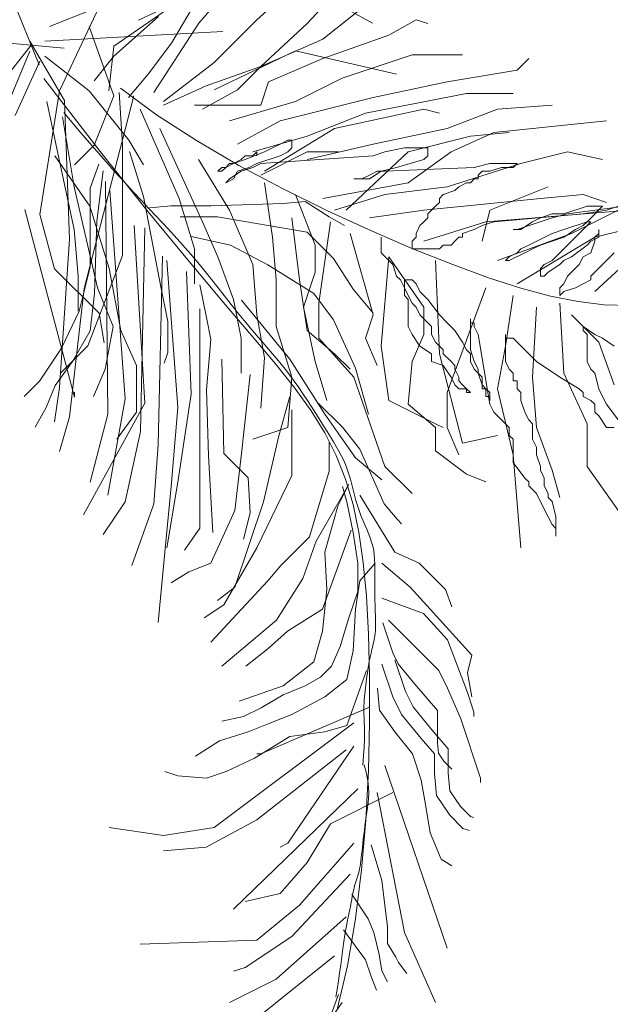
# Model space of a CAD drawing. Units: millimetres. Extents: x 595116 to 630915, y 909473 to 920225.
# Tile 98 of 134: x 629805.265 to 629809.617, y 919164.766 to 919172.019. Entities that reach past the tile are written whole.
import ezdxf

# ---------------------------------------------------------------- set-up
doc = ezdxf.new("R2010")
doc.units = ezdxf.units.MM
doc.layers.add('L-PLNT', color=85, linetype='Continuous', lineweight=13)

# ---------------------------------------------------------------- blocks, each defined once
blk = doc.blocks.new('A$C4FB75ABC')
for p, q in [((2.6324, 2.4053), (2.7073, 2.2214)), ((3.0207, 2.3031), (3.1093, 2.4053)), ((3.1344, 2.3096), (3.2259, 2.3934)), ((3.2335, 2.302), (3.3174, 2.3934)), ((2.7277, 2.2964), (2.8733, 2.3546)), ((2.8539, 2.2576), (2.9801, 2.3449)), ((2.9022, 2.3089), (3.0036, 2.3566)), ((2.9666, 2.2638), (3.0123, 2.3401)), ((2.8248, 2.3352), (2.7471, 2.1703)), ((3.264, 2.2715), (3.3403, 2.3324)), ((3.3079, 2.3327), (3.3615, 2.3029)), ((2.8539, 2.2382), (2.9413, 2.3158)), ((2.9321, 2.167), (3.0207, 2.3031)), ((3.0505, 2.2257), (3.1344, 2.3096)), ((3.142, 2.2181), (3.2335, 2.302)), ((3.3937, 2.2791), (3.447, 2.3096)), ((3.447, 2.3096), (3.4699, 2.302)), ((2.718, 2.2673), (3.0675, 2.2867)), ((2.8054, 2.2964), (2.8539, 2.1606)), ((2.6937, 2.2623), (2.4825, 1.9967)), ((2.7559, 2.2536), (2.4852, 2.2785)), ((2.6889, 2.2673), (2.7568, 2.1509)), ((2.9208, 2.2029), (2.9666, 2.2638)), ((3.142, 2.2181), (3.264, 2.2715)), ((3.264, 2.2334), (3.3937, 2.2791)), ((2.6889, 2.2479), (2.6404, 2.1315)), ((2.8442, 2.1703), (2.8539, 2.2576)), ((3.0505, 2.1724), (3.2106, 2.2486)), ((3.2106, 2.2486), (3.4089, 2.2029)), ((2.7083, 2.2285), (2.6598, 2.1218)), ((2.718, 2.2382), (2.8054, 2.1703)), ((2.8151, 2.1897), (2.8539, 2.2382)), ((2.9513, 2.1495), (3.0505, 2.2257)), ((3.1572, 2.1876), (3.264, 2.2334)), ((3.3021, 2.1952), (3.4394, 2.241)), ((3.4394, 2.241), (3.5385, 2.241)), ((3.6453, 2.2105), (3.6682, 2.2334)), ((3.0352, 2.18), (3.142, 2.2181)), ((3.0962, 2.1724), (3.142, 2.2181)), ((3.508, 2.1876), (3.6453, 2.2105)), ((2.7162, 2.1941), (2.8268, 2.0511)), ((2.8827, 2.1571), (2.9208, 2.2029)), ((3.142, 2.1419), (3.1572, 2.1876)), ((3.2106, 2.1495), (3.3021, 2.1952)), ((3.3631, 2.1571), (3.508, 2.1876)), ((2.7471, 2.1703), (2.7083, 1.9277)), ((2.8054, 2.1703), (2.883, 2.0733)), ((2.864, 2.167), (2.8708, 2.0648)), ((2.9375, 2.1232), (2.8667, 2.1755)), ((2.9513, 2.1419), (3.0352, 2.18)), ((3.0276, 2.1343), (3.0962, 2.1724)), ((3.3479, 2.1266), (3.5462, 2.1648)), ((3.5462, 2.1648), (3.6377, 2.1648)), ((2.7225, 2.1495), (2.753, 2.0047)), ((2.7568, 2.1509), (2.7666, 1.8792)), ((2.8927, 2.1606), (2.7957, 1.7822)), ((2.8539, 2.1606), (2.8151, 2.0636)), ((3.081, 2.1114), (3.2106, 2.1495)), ((3.1801, 2.1114), (3.3631, 2.1571)), ((2.7555, 2.1274), (2.7844, 2.0931)), ((2.9056, 2.1343), (2.9818, 1.9589)), ((3.0123, 2.1419), (3.142, 2.1419)), ((3.2335, 2.0809), (3.3479, 2.1266)), ((3.2869, 2.0961), (3.4623, 2.1343)), ((3.4623, 2.1343), (3.4928, 2.1266)), ((3.508, 2.0961), (3.6072, 2.1343)), ((3.6072, 2.1343), (3.714, 2.1419)), ((2.753, 2.119), (2.7759, 1.9818)), ((3.0158, 2.0725), (2.9375, 2.1232)), ((3.0962, 2.0657), (3.1801, 2.1114)), ((3.5996, 2.0885), (3.8207, 2.1114)), ((2.7844, 2.0931), (2.8104, 2.0628)), ((2.9437, 2.0961), (3.0276, 1.9132)), ((3.1496, 2.0123), (3.2869, 2.0961)), ((3.3631, 2.0657), (3.508, 2.0961)), ((3.5157, 2.0504), (3.5996, 2.0885)), ((3.5538, 2.0809), (3.6301, 2.0885)), ((2.883, 2.0733), (2.9122, 2.0248)), ((3.0992, 2.0238), (3.0158, 2.0725)), ((3.1267, 2.0504), (3.2335, 2.0809)), ((3.1954, 2.0733), (3.1801, 2.0657)), ((3.203, 2.0733), (3.1954, 2.0733)), ((3.203, 2.058), (3.203, 2.0733)), ((3.4318, 2.0504), (3.5538, 2.0809)), ((2.8151, 2.0636), (2.7763, 2.0248)), ((2.8104, 2.0628), (2.8339, 2.0359)), ((2.8268, 2.0511), (2.9214, 1.9326)), ((2.8708, 2.0648), (2.8708, 1.8469)), ((2.8844, 2.0512), (2.9117, 1.9627)), ((3.1496, 2.0504), (3.1115, 2.0352)), ((3.1267, 2.0428), (3.1344, 2.0504)), ((3.1344, 2.0504), (3.1344, 2.0428)), ((3.142, 2.0047), (3.2335, 2.0504)), ((3.1649, 2.058), (3.1496, 2.0504)), ((3.1801, 2.0657), (3.1649, 2.058)), ((3.1801, 2.0428), (3.1954, 2.0504)), ((3.1954, 2.0504), (3.203, 2.058)), ((3.2335, 2.0352), (3.3631, 2.0657)), ((3.2335, 2.0504), (3.2945, 2.0504)), ((3.3098, 1.9361), (3.4318, 2.0504)), ((3.386, 2.0504), (3.3631, 2.0428)), ((3.4242, 2.058), (3.386, 2.0504)), ((3.4699, 2.058), (3.4242, 2.058)), ((3.4318, 1.9894), (3.5157, 2.0504)), ((3.4699, 2.0428), (3.4699, 2.058)), ((3.6529, 2.0275), (3.7445, 2.0504)), ((3.7445, 2.0504), (3.8131, 2.0352)), ((2.7378, 2.0428), (2.8064, 1.9437)), ((2.8339, 2.0359), (2.8551, 2.0121)), ((3.02, 2.0352), (3.081, 1.9361)), ((3.1115, 2.0352), (3.0886, 2.0275)), ((3.0886, 2.0275), (3.1039, 2.0352)), ((3.1039, 2.0352), (3.1115, 2.0428)), ((3.1115, 2.0428), (3.1267, 2.0428)), ((3.1344, 2.0275), (3.1801, 2.0428)), ((3.3631, 2.0428), (3.142, 2.0275)), ((3.4089, 2.0199), (3.4623, 2.0352)), ((3.4623, 2.0352), (3.4699, 2.0428)), ((2.8244, 2.0263), (2.8071, 1.979)), ((2.833, 2.0134), (2.8201, 1.9144)), ((2.8551, 2.0121), (2.8744, 1.9909)), ((3.0581, 2.0123), (3.0657, 2.0199)), ((3.0657, 2.0123), (3.0581, 2.0123)), ((3.0734, 2.0199), (3.0657, 2.0123)), ((3.0657, 2.0199), (3.0734, 2.0199)), ((3.0734, 2.0199), (3.081, 2.0275)), ((3.0886, 2.0275), (3.0734, 2.0199)), ((3.081, 2.0275), (3.0886, 2.0275)), ((3.1039, 2.0123), (3.081, 1.9971)), ((3.0886, 1.9971), (3.0962, 2.0123)), ((3.0962, 2.0123), (3.1191, 2.0199)), ((3.1858, 1.9776), (3.0992, 2.0238)), ((3.1267, 2.0199), (3.1039, 2.0123)), ((3.1191, 2.0199), (3.1344, 2.0275)), ((3.142, 2.0275), (3.1267, 2.0199)), ((3.3708, 2.0123), (3.3555, 2.0047)), ((3.3555, 1.9971), (3.3784, 2.0123)), ((3.386, 2.0123), (3.3708, 2.0123)), ((3.3784, 2.0123), (3.4089, 2.0199)), ((3.5614, 2.0199), (3.386, 2.0123)), ((3.508, 1.9818), (3.6529, 2.0275)), ((3.5919, 2.0275), (3.5614, 2.0199)), ((3.5691, 2.0047), (3.5767, 2.0123)), ((3.5767, 2.0123), (3.5919, 2.0123)), ((3.6453, 2.0275), (3.5919, 2.0275)), ((3.5919, 2.0123), (3.6148, 2.0199)), ((3.6148, 2.0199), (3.6377, 2.0199)), ((3.6377, 2.0199), (3.6453, 2.0275)), ((2.753, 2.0047), (2.7759, 1.898)), ((2.8373, 1.9919), (2.8416, 1.5357)), ((2.8744, 1.9909), (2.8918, 1.9721)), ((3.081, 1.9971), (3.0734, 1.9894)), ((3.0734, 1.9894), (3.0886, 1.9971)), ((3.3403, 1.9971), (3.325, 1.9971)), ((3.325, 1.9971), (3.3555, 1.9971)), ((3.3555, 2.0047), (3.3403, 1.9971)), ((3.5538, 1.9894), (3.5614, 1.9971)), ((3.5614, 1.9971), (3.5691, 1.9971)), ((3.5691, 1.9971), (3.5691, 2.0047)), ((2.7759, 1.9818), (2.8217, 1.7836)), ((2.8071, 1.979), (2.8071, 1.9015)), ((2.8459, 1.9747), (2.876, 1.5659)), ((2.8918, 1.9721), (2.9078, 1.955)), ((3.1496, 1.9894), (3.1649, 1.8827)), ((3.2732, 1.9345), (3.1858, 1.9776)), ((3.264, 1.9589), (3.4318, 1.9894)), ((3.386, 1.9666), (3.508, 1.9818)), ((3.5004, 1.9666), (3.5233, 1.9742)), ((3.5233, 1.9742), (3.5309, 1.9818)), ((3.5309, 1.9818), (3.5462, 1.9894)), ((3.5462, 1.9894), (3.5538, 1.9894)), ((3.5919, 1.9361), (3.7063, 1.9818)), ((2.9078, 1.955), (2.9225, 1.9395)), ((2.9117, 1.9627), (2.9458, 1.7856)), ((2.9818, 1.9589), (3.0123, 1.8599)), ((3.186, 1.9488), (3.2291, 1.9531)), ((3.2106, 1.9666), (3.2488, 1.8675)), ((3.2291, 1.9531), (3.2764, 1.923)), ((3.2869, 1.9361), (3.386, 1.9666)), ((3.4623, 1.9361), (3.6911, 1.9589)), ((3.4928, 1.9589), (3.5004, 1.9666)), ((3.4928, 1.9513), (3.4928, 1.9589)), ((3.6911, 1.9589), (3.775, 1.9666)), ((3.7521, 1.8903), (3.8894, 1.9589)), ((3.775, 1.9666), (3.8207, 1.9513)), ((2.6792, 1.9375), (2.7763, 1.5688)), ((2.8064, 1.9437), (2.8446, 1.8217)), ((2.9214, 1.9326), (3.0014, 1.8351)), ((2.9225, 1.9395), (2.9361, 1.925)), ((2.9234, 1.9402), (2.9664, 1.9445)), ((2.9664, 1.9445), (3.0439, 1.9445)), ((3.0439, 1.9445), (3.186, 1.9488)), ((3.081, 1.9361), (3.1267, 1.8294)), ((3.3593, 1.8951), (3.2732, 1.9345)), ((3.3555, 1.9208), (3.4623, 1.9361)), ((3.4699, 1.9285), (3.4852, 1.9437)), ((3.4852, 1.9437), (3.4928, 1.9513)), ((3.5767, 1.8751), (3.5919, 1.9361)), ((3.5843, 1.9132), (3.8665, 1.9361)), ((3.7826, 1.9437), (3.7368, 1.9285)), ((3.7445, 1.9285), (3.9122, 1.9513)), ((3.8207, 1.9361), (3.775, 1.9285)), ((3.7826, 1.9132), (3.8131, 1.9437)), ((3.8131, 1.9437), (3.7826, 1.9437)), ((3.7978, 1.8827), (4.0495, 1.9437)), ((3.8665, 1.9513), (3.8207, 1.9361)), ((2.7083, 1.9277), (2.7374, 1.821)), ((2.8201, 1.9144), (2.8158, 1.7724)), ((2.9361, 1.925), (2.9489, 1.9114)), ((2.9837, 1.923), (3.0569, 1.923)), ((3.0276, 1.9132), (3.0581, 1.8446)), ((3.0569, 1.923), (3.2334, 1.8929)), ((3.203, 1.9208), (3.2182, 1.7989)), ((3.2793, 1.9132), (3.2564, 1.7531)), ((3.2764, 1.923), (3.3066, 1.9058)), ((3.4547, 1.9056), (3.4623, 1.9132)), ((3.4623, 1.9132), (3.4699, 1.9208)), ((3.4623, 1.8751), (3.5843, 1.9132)), ((3.4699, 1.9208), (3.4699, 1.9285)), ((3.5996, 1.9132), (3.5767, 1.9056)), ((3.775, 1.9285), (3.5996, 1.9132)), ((3.6453, 1.898), (3.714, 1.9208)), ((3.6758, 1.9132), (3.6529, 1.898)), ((3.6911, 1.9208), (3.6758, 1.9132)), ((3.714, 1.9285), (3.6911, 1.9208)), ((3.7368, 1.9285), (3.714, 1.9285)), ((3.714, 1.9208), (3.7445, 1.9285)), ((3.7368, 1.898), (3.7826, 1.9132)), ((3.7826, 1.9132), (3.775, 1.9056)), ((3.7826, 1.9056), (3.7902, 1.9132)), ((3.7902, 1.9132), (3.7826, 1.9132)), ((2.7759, 1.898), (2.7836, 1.8065)), ((2.8071, 1.9015), (2.8071, 1.8241)), ((2.8933, 1.9058), (2.9148, 1.5573)), ((2.9148, 1.9015), (2.9062, 1.5013)), ((2.9489, 1.9114), (2.9609, 1.8985)), ((2.9609, 1.8985), (2.9724, 1.8861)), ((3.4421, 1.8597), (3.3593, 1.8951)), ((3.447, 1.8903), (3.4547, 1.9056)), ((3.5614, 1.898), (3.5385, 1.8903)), ((3.5767, 1.9056), (3.5614, 1.898)), ((3.6529, 1.898), (3.6377, 1.898)), ((3.6377, 1.898), (3.6453, 1.898)), ((3.714, 1.8903), (3.7368, 1.898)), ((3.7597, 1.898), (3.7368, 1.8827)), ((3.7597, 1.8827), (3.7826, 1.9056)), ((3.775, 1.9056), (3.7597, 1.898)), ((3.8055, 1.8903), (3.8055, 1.898)), ((3.8055, 1.898), (3.8055, 1.8827)), ((2.7666, 1.8792), (2.7471, 1.5882)), ((2.9724, 1.8861), (2.9834, 1.874)), ((3.0052, 1.8843), (3.0827, 1.8671)), ((3.1649, 1.8827), (3.1725, 1.7989)), ((3.2334, 1.8929), (3.285, 1.8413)), ((3.3174, 1.8903), (3.3631, 1.7303)), ((3.3784, 1.8827), (3.3784, 1.8522)), ((3.4394, 1.8751), (3.447, 1.8827)), ((3.4394, 1.8599), (3.4394, 1.8751)), ((3.447, 1.8827), (3.447, 1.8903)), ((3.5233, 1.8751), (3.5157, 1.8675)), ((3.5309, 1.8827), (3.5233, 1.8751)), ((3.5385, 1.8827), (3.5309, 1.8827)), ((3.5385, 1.8903), (3.5385, 1.8827)), ((3.6072, 1.837), (3.7521, 1.8903)), ((3.6453, 1.7913), (3.7978, 1.8827)), ((3.6682, 1.8675), (3.714, 1.8903)), ((3.7368, 1.8827), (3.6911, 1.8675)), ((3.7368, 1.8599), (3.7521, 1.8751)), ((3.7521, 1.8751), (3.7597, 1.8827)), ((3.7902, 1.8751), (3.7826, 1.8675)), ((3.8055, 1.8827), (3.7902, 1.8751)), ((3.7902, 1.8522), (3.7978, 1.8751)), ((3.7978, 1.8827), (3.8055, 1.8903)), ((3.7978, 1.8751), (3.7978, 1.8827)), ((2.9834, 1.874), (2.994, 1.862)), ((2.994, 1.862), (3.0045, 1.8499)), ((3.0123, 1.8599), (3.0123, 1.7913)), ((3.0827, 1.8671), (3.1559, 1.8284)), ((3.2488, 1.8675), (3.2488, 1.8141)), ((3.4928, 1.8599), (3.4394, 1.8599)), ((3.5192, 1.829), (3.4421, 1.8597)), ((3.5004, 1.8675), (3.4928, 1.8599)), ((3.5157, 1.8675), (3.5004, 1.8675)), ((3.6453, 1.8522), (3.6529, 1.8599)), ((3.6529, 1.8599), (3.6682, 1.8675)), ((3.6758, 1.8599), (3.6606, 1.8522)), ((3.6911, 1.8675), (3.6758, 1.8599)), ((3.714, 1.837), (3.7368, 1.8599)), ((3.7826, 1.8675), (3.7521, 1.8446)), ((3.7978, 1.776), (3.897, 1.8675)), ((2.8708, 1.8469), (2.8027, 1.6699)), ((2.9492, 1.8456), (2.9406, 1.4755)), ((2.9578, 1.837), (2.9794, 1.5486)), ((3.0045, 1.8499), (3.0149, 1.8377)), ((3.0149, 1.8377), (3.0253, 1.8251)), ((3.0581, 1.8446), (3.0886, 1.7608)), ((3.285, 1.8413), (3.3238, 1.781)), ((3.3784, 1.8522), (3.3937, 1.837)), ((3.3937, 1.8446), (3.3784, 1.6693)), ((3.3937, 1.8446), (3.4623, 1.7455)), ((3.3937, 1.837), (3.4013, 1.8294)), ((3.4852, 1.837), (3.4928, 1.6541)), ((3.6224, 1.837), (3.6301, 1.8446)), ((3.6301, 1.837), (3.6224, 1.837)), ((3.6606, 1.8522), (3.6301, 1.837)), ((3.6301, 1.8446), (3.6453, 1.8522)), ((3.6987, 1.8294), (3.714, 1.837)), ((3.7368, 1.837), (3.7292, 1.8294)), ((3.7521, 1.8446), (3.7368, 1.837)), ((3.7673, 1.8294), (3.775, 1.8446)), ((3.775, 1.8446), (3.7902, 1.8522)), ((3.8207, 1.837), (3.8131, 1.8294)), ((3.836, 1.8522), (3.8207, 1.837)), ((2.7374, 1.821), (2.8248, 1.7337)), ((2.8071, 1.8241), (2.7856, 1.738)), ((2.8446, 1.8217), (2.8674, 1.6998)), ((3.0014, 1.8351), (3.0686, 1.7552)), ((3.0253, 1.8251), (3.0358, 1.8122)), ((3.1267, 1.8294), (3.1344, 1.7303)), ((3.1559, 1.8284), (3.2463, 1.7724)), ((3.4013, 1.8294), (3.4089, 1.8065)), ((3.5892, 1.8034), (3.5192, 1.829)), ((3.6911, 1.8217), (3.6987, 1.8294)), ((3.6911, 1.8065), (3.6911, 1.8217)), ((3.7292, 1.8294), (3.7063, 1.8141)), ((3.7445, 1.8065), (3.7673, 1.8294)), ((3.8131, 1.8294), (3.7902, 1.8065)), ((2.7836, 1.8065), (2.7836, 1.7379)), ((2.9966, 1.8154), (3.0052, 1.5745)), ((3.0358, 1.8122), (3.0461, 1.7993)), ((3.0461, 1.7993), (3.0562, 1.7866)), ((3.1725, 1.7989), (3.1725, 1.7074)), ((3.2182, 1.7989), (3.2335, 1.6998)), ((3.2488, 1.8141), (3.2259, 1.7455)), ((3.4089, 1.8065), (3.4165, 1.7989)), ((3.4165, 1.7989), (3.4242, 1.7836)), ((3.4242, 1.7684), (3.4242, 1.7989)), ((3.4242, 1.7989), (3.4394, 1.7989)), ((3.4394, 1.7989), (3.447, 1.7913)), ((3.6527, 1.7828), (3.5892, 1.8034)), ((3.6987, 1.8065), (3.6911, 1.8065)), ((3.7063, 1.8141), (3.6987, 1.8065)), ((3.7368, 1.7913), (3.7445, 1.8065)), ((3.7902, 1.7989), (3.775, 1.7913)), ((3.7902, 1.8065), (3.7902, 1.7989)), ((2.7957, 1.7822), (2.7666, 1.53)), ((2.8217, 1.7836), (2.8522, 1.7074)), ((2.9458, 1.7856), (2.9594, 1.7175)), ((3.0224, 1.7896), (3.0353, 1.7251)), ((3.0562, 1.7866), (3.0659, 1.7741)), ((3.3238, 1.781), (3.3625, 1.7337)), ((3.4242, 1.7836), (3.4318, 1.7684)), ((3.447, 1.7913), (3.4547, 1.776)), ((3.5843, 1.7836), (3.508, 1.5778)), ((3.7109, 1.7672), (3.6527, 1.7828)), ((3.7292, 1.7836), (3.7368, 1.7913)), ((3.7292, 1.7684), (3.7292, 1.7836)), ((3.7597, 1.7836), (3.7368, 1.776)), ((3.775, 1.7913), (3.7597, 1.7836)), ((2.8158, 1.7724), (2.8071, 1.6993)), ((3.0659, 1.7741), (3.0752, 1.7623)), ((3.0752, 1.7623), (3.084, 1.7511)), ((3.0886, 1.7608), (3.1039, 1.6845)), ((3.1042, 1.7595), (3.1989, 1.6433)), ((3.2463, 1.7724), (3.285, 1.7208)), ((3.4318, 1.7608), (3.4242, 1.7684)), ((3.4318, 1.7684), (3.4394, 1.7531)), ((3.4318, 1.7074), (3.4318, 1.7608)), ((3.4547, 1.776), (3.4699, 1.7608)), ((3.4699, 1.7608), (3.4928, 1.7303)), ((3.6377, 1.7684), (3.6224, 1.6693)), ((3.7651, 1.7564), (3.7109, 1.7672)), ((3.7368, 1.776), (3.7292, 1.7684)), ((3.0224, 1.7423), (3.0224, 1.312)), ((3.0686, 1.7552), (3.1246, 1.6894)), ((3.084, 1.7511), (3.0921, 1.7408)), ((3.0921, 1.7408), (3.0994, 1.7316)), ((3.2259, 1.7455), (3.2488, 1.6388)), ((3.2564, 1.7531), (3.2564, 1.6845)), ((3.4394, 1.7531), (3.447, 1.7455)), ((3.447, 1.7455), (3.4547, 1.7303)), ((3.4623, 1.7455), (3.4623, 1.6922)), ((3.6834, 1.7455), (3.6758, 1.6083)), ((3.7292, 1.7531), (3.7368, 1.6159)), ((3.8165, 1.7504), (3.7651, 1.7564)), ((3.8664, 1.749), (3.8165, 1.7504)), ((2.7856, 1.738), (2.7512, 1.6648)), ((2.8248, 1.7337), (2.8345, 1.6755)), ((3.0353, 1.7251), (3.0439, 1.682)), ((3.0994, 1.7316), (3.1062, 1.7232)), ((3.1062, 1.7232), (3.1126, 1.7155)), ((3.1344, 1.7303), (3.1496, 1.6464)), ((3.285, 1.7208), (3.3281, 1.6261)), ((3.3631, 1.7303), (3.3479, 1.6845)), ((3.4547, 1.7303), (3.4699, 1.715)), ((3.4928, 1.7303), (3.508, 1.715)), ((3.5538, 1.7227), (3.5538, 1.715)), ((3.5538, 1.6617), (3.5538, 1.7227)), ((3.7521, 1.7303), (3.8055, 1.6769)), ((2.8522, 1.7074), (2.8369, 1.6236)), ((2.9594, 1.7175), (2.9594, 1.6563)), ((3.1126, 1.7155), (3.1186, 1.7083)), ((3.1186, 1.7083), (3.1246, 1.7013)), ((3.1246, 1.7013), (3.1305, 1.6944)), ((3.1725, 1.7074), (3.203, 1.6083)), ((3.4394, 1.6922), (3.4318, 1.7074)), ((3.4699, 1.715), (3.4775, 1.7074)), ((3.4775, 1.7074), (3.4775, 1.6922)), ((3.508, 1.715), (3.5233, 1.6998)), ((3.5538, 1.715), (3.5614, 1.715)), ((3.5614, 1.715), (3.5614, 1.7074)), ((3.5614, 1.7074), (3.5691, 1.6922)), ((3.775, 1.6998), (3.775, 1.7074)), ((3.775, 1.7074), (3.7978, 1.6922)), ((2.8071, 1.6993), (2.7727, 1.639)), ((2.8674, 1.6998), (2.8979, 1.6312)), ((3.0439, 1.682), (3.0353, 1.5831)), ((3.1039, 1.6845), (3.1039, 1.6159)), ((3.1246, 1.6894), (3.1709, 1.6342)), ((3.1305, 1.6944), (3.1367, 1.6873)), ((3.1367, 1.6873), (3.1432, 1.6798)), ((3.2335, 1.6998), (3.2869, 1.6541)), ((3.2564, 1.6845), (3.325, 1.6083)), ((3.3479, 1.6845), (3.3708, 1.6312)), ((3.4547, 1.6693), (3.4394, 1.6922)), ((3.4623, 1.6922), (3.4394, 1.6388)), ((3.4775, 1.6922), (3.4852, 1.6769)), ((3.5233, 1.6998), (3.5385, 1.6769)), ((3.5691, 1.6922), (3.5919, 1.555)), ((3.6224, 1.6922), (3.6224, 1.6845)), ((3.6224, 1.6388), (3.6224, 1.6922)), ((3.6224, 1.6845), (3.6377, 1.6845)), ((3.6377, 1.6845), (3.6453, 1.6769)), ((3.7826, 1.6922), (3.775, 1.6998)), ((3.7826, 1.6388), (3.7826, 1.6922)), ((3.7978, 1.6922), (3.8131, 1.6845)), ((3.8131, 1.6845), (3.836, 1.6693)), ((2.7512, 1.6648), (2.7081, 1.6003)), ((2.8027, 1.6699), (2.7482, 1.6154)), ((3.1432, 1.6798), (3.1502, 1.6718)), ((3.1502, 1.6718), (3.1576, 1.6632)), ((3.1576, 1.6632), (3.1654, 1.654)), ((3.3784, 1.6693), (3.3937, 1.5626)), ((3.4775, 1.6541), (3.4547, 1.6693)), ((3.4852, 1.6769), (3.4928, 1.6693)), ((3.4928, 1.6693), (3.5004, 1.6617)), ((3.5385, 1.6769), (3.5462, 1.6617)), ((3.6224, 1.6693), (3.6072, 1.5855)), ((3.6453, 1.6769), (3.6682, 1.6541)), ((3.8055, 1.6769), (3.836, 1.5931)), ((2.9594, 1.6563), (2.9526, 1.6358)), ((3.0655, 1.6433), (3.0698, 1.4583)), ((3.1496, 1.6464), (3.142, 1.5473)), ((3.1654, 1.654), (3.1735, 1.6443)), ((3.1735, 1.6443), (3.1819, 1.634)), ((3.1989, 1.6433), (3.2678, 1.5357)), ((3.2869, 1.6541), (3.3174, 1.6236)), ((3.4775, 1.6388), (3.4775, 1.6541)), ((3.4928, 1.6541), (3.5385, 1.4787)), ((3.5004, 1.6617), (3.5004, 1.6541)), ((3.5004, 1.6541), (3.5157, 1.6388)), ((3.5462, 1.6617), (3.5538, 1.6541)), ((3.5614, 1.6388), (3.5538, 1.6617)), ((3.5538, 1.6541), (3.5538, 1.6388)), ((3.6682, 1.6541), (3.6834, 1.6388)), ((2.7727, 1.639), (2.7383, 1.5917)), ((2.8369, 1.6236), (2.8141, 1.5702)), ((2.8979, 1.6312), (2.8979, 1.5397)), ((3.1709, 1.6342), (3.2091, 1.5863)), ((3.1819, 1.634), (3.1904, 1.6232)), ((3.2488, 1.6388), (3.2716, 1.5626)), ((3.3281, 1.6261), (3.3539, 1.5357)), ((3.4394, 1.6388), (3.4318, 1.555)), ((3.5004, 1.6312), (3.4775, 1.6388)), ((3.5157, 1.6083), (3.5004, 1.6312)), ((3.5157, 1.6388), (3.5233, 1.6312)), ((3.5233, 1.6312), (3.5233, 1.6236)), ((3.5233, 1.6236), (3.5309, 1.6083)), ((3.5538, 1.6388), (3.5614, 1.6236)), ((3.5691, 1.6236), (3.5614, 1.6388)), ((3.5614, 1.6236), (3.5691, 1.6159)), ((3.5691, 1.6159), (3.5691, 1.6236)), ((3.6301, 1.6236), (3.6224, 1.6388)), ((3.6377, 1.6159), (3.6301, 1.6236)), ((3.6834, 1.6388), (3.7292, 1.6083)), ((3.7902, 1.6236), (3.7826, 1.6388)), ((3.7978, 1.6159), (3.7902, 1.6236)), ((3.1214, 1.6132), (3.1042, 1.4583)), ((3.1904, 1.6232), (3.1991, 1.6119)), ((3.203, 1.6083), (3.1954, 1.5092)), ((3.1991, 1.6119), (3.2078, 1.6)), ((3.325, 1.6083), (3.386, 1.433)), ((3.5233, 1.5931), (3.5157, 1.6083)), ((3.5309, 1.6083), (3.5309, 1.6007)), ((3.5691, 1.6159), (3.5767, 1.6083)), ((3.5767, 1.5931), (3.5691, 1.6159)), ((3.5767, 1.6083), (3.5767, 1.5855)), ((3.6377, 1.6007), (3.6377, 1.6159)), ((3.6758, 1.6083), (3.6834, 1.5092)), ((3.7292, 1.6083), (3.7673, 1.5855)), ((3.7368, 1.6159), (3.7826, 1.5168)), ((3.8055, 1.5855), (3.7978, 1.6159)), ((2.7081, 1.6003), (2.678, 1.5702)), ((2.7383, 1.5917), (2.721, 1.5486)), ((2.7471, 1.5882), (2.7374, 1.5203)), ((3.2078, 1.6), (3.2166, 1.5877)), ((3.2091, 1.5863), (3.241, 1.5422)), ((3.2166, 1.5877), (3.2252, 1.575)), ((3.5309, 1.5855), (3.5233, 1.5931)), ((3.5309, 1.6007), (3.5385, 1.5931)), ((3.5462, 1.5855), (3.5309, 1.5855)), ((3.5385, 1.5931), (3.5462, 1.5855)), ((3.5462, 1.5855), (3.5462, 1.5778)), ((3.5538, 1.5778), (3.5462, 1.5855)), ((3.5843, 1.5855), (3.5767, 1.5931)), ((3.5767, 1.5855), (3.5843, 1.5855)), ((3.5843, 1.5855), (3.5843, 1.5702)), ((3.5919, 1.5778), (3.5843, 1.5855)), ((3.6072, 1.5855), (3.6377, 1.4559)), ((3.6453, 1.6007), (3.6377, 1.6007)), ((3.6453, 1.5855), (3.6453, 1.6007)), ((3.6529, 1.5778), (3.6453, 1.5855)), ((3.7673, 1.5855), (3.775, 1.5778)), ((3.8131, 1.5702), (3.8055, 1.5855)), ((2.7763, 1.5688), (2.7763, 1.5785)), ((2.876, 1.5659), (2.8416, 1.3765)), ((3.0052, 1.5745), (2.9794, 1.4023)), ((3.0353, 1.5831), (3.0396, 1.454)), ((3.1989, 1.5702), (3.1774, 1.4927)), ((3.2252, 1.575), (3.2338, 1.5622)), ((3.508, 1.5778), (3.508, 1.5092)), ((3.5462, 1.5778), (3.5538, 1.5778)), ((3.5843, 1.5702), (3.5919, 1.5702)), ((3.5919, 1.5626), (3.5919, 1.5778)), ((3.5919, 1.5702), (3.5919, 1.5626)), ((3.6529, 1.5626), (3.6529, 1.5778)), ((3.775, 1.5778), (3.775, 1.5702)), ((3.775, 1.5702), (3.7902, 1.5626)), ((3.8207, 1.555), (3.8131, 1.5702)), ((2.721, 1.5486), (2.6995, 1.5099)), ((2.9148, 1.5573), (2.7942, 1.3378)), ((2.9794, 1.5486), (2.9664, 1.3937)), ((3.2338, 1.5622), (3.2421, 1.5493)), ((3.2421, 1.5493), (3.2503, 1.5367)), ((3.2549, 1.5573), (3.3023, 1.5099)), ((3.3937, 1.5626), (3.4852, 1.5168)), ((3.4318, 1.555), (3.4852, 1.5092)), ((3.5919, 1.555), (3.5996, 1.5397)), ((3.6606, 1.5397), (3.6529, 1.5626)), ((3.7902, 1.5626), (3.7978, 1.555)), ((3.7978, 1.555), (3.7978, 1.5397)), ((3.8436, 1.5245), (3.8207, 1.555)), ((2.7666, 1.53), (2.7471, 1.462)), ((2.8416, 1.5357), (2.8071, 1.4023)), ((2.8979, 1.5397), (2.8598, 1.4864)), ((3.2032, 1.5443), (3.2032, 1.4152)), ((3.241, 1.5422), (3.2678, 1.4987)), ((3.2503, 1.5367), (3.258, 1.5243)), ((3.2678, 1.5357), (3.3281, 1.4497)), ((3.5996, 1.5397), (3.6301, 1.5092)), ((3.6682, 1.5245), (3.6606, 1.5397)), ((3.7978, 1.5397), (3.8055, 1.5321)), ((3.8055, 1.5321), (3.8207, 1.5092)), ((3.1954, 1.5092), (3.1267, 1.4864)), ((3.258, 1.5243), (3.2655, 1.5125)), ((3.2655, 1.5125), (3.2724, 1.5013)), ((3.3023, 1.5099), (3.3367, 1.4669)), ((3.4852, 1.5168), (3.5004, 1.5092)), ((3.4852, 1.5092), (3.4852, 1.4635)), ((3.508, 1.5092), (3.5309, 1.4559)), ((3.6301, 1.5092), (3.6301, 1.494)), ((3.6758, 1.5168), (3.6682, 1.5245)), ((3.6758, 1.4864), (3.6758, 1.5168)), ((3.6834, 1.5092), (3.714, 1.4254)), ((3.7826, 1.5168), (3.7826, 1.433)), ((3.8207, 1.5092), (3.836, 1.5092)), ((2.9062, 1.5013), (2.876, 1.3636)), ((3.1774, 1.4927), (3.1473, 1.3636)), ((3.2678, 1.4987), (3.2902, 1.4543)), ((3.2724, 1.5013), (3.2789, 1.491)), ((3.2789, 1.491), (3.2849, 1.4813)), ((3.5385, 1.4787), (3.6072, 1.494)), ((3.6301, 1.494), (3.6377, 1.4864)), ((2.9406, 1.4755), (2.932, 1.3593)), ((3.2764, 1.4798), (3.2764, 1.4239)), ((3.2849, 1.4813), (3.2904, 1.4721)), ((3.2904, 1.4721), (3.2955, 1.4632)), ((3.6377, 1.4864), (3.6377, 1.4406)), ((3.6834, 1.4711), (3.6758, 1.4864)), ((3.6834, 1.4559), (3.6834, 1.4711)), ((3.0396, 1.454), (3.0483, 1.3034)), ((3.0698, 1.4583), (3.1171, 1.4109)), ((3.1042, 1.4583), (3.0913, 1.3464)), ((3.2902, 1.4543), (3.3086, 1.4079)), ((3.2955, 1.4632), (3.3002, 1.4545)), ((3.3002, 1.4545), (3.3045, 1.4458)), ((3.3281, 1.4497), (3.3798, 1.4066)), ((3.3367, 1.4669), (3.3841, 1.3593)), ((3.4852, 1.4635), (3.5462, 1.4178)), ((3.6377, 1.4559), (3.6529, 1.2729)), ((3.6911, 1.433), (3.6834, 1.4559)), ((3.3045, 1.4458), (3.3084, 1.437)), ((3.3084, 1.437), (3.3119, 1.4278)), ((3.386, 1.433), (3.4394, 1.3796)), ((3.6377, 1.4406), (3.6606, 1.4101)), ((3.6911, 1.4254), (3.6911, 1.433)), ((3.7826, 1.433), (3.8741, 1.3034)), ((3.1171, 1.4109), (3.1214, 1.3421)), ((3.2032, 1.4152), (3.1344, 1.2732)), ((3.2764, 1.4239), (3.2377, 1.2948)), ((3.3119, 1.4278), (3.3151, 1.4181)), ((3.3151, 1.4181), (3.3181, 1.4081)), ((3.5462, 1.4178), (3.5843, 1.4025)), ((3.6987, 1.4101), (3.6911, 1.4254)), ((3.714, 1.4254), (3.7292, 1.372)), ((2.9664, 1.3937), (2.9535, 1.2646)), ((2.9794, 1.4023), (2.9578, 1.2732)), ((3.2937, 1.355), (3.3152, 1.398)), ((3.298, 1.3679), (3.3152, 1.398)), ((3.3023, 1.3937), (3.3109, 1.3636)), ((3.3086, 1.4079), (3.3233, 1.3583)), ((3.3181, 1.4081), (3.3209, 1.3978)), ((3.3209, 1.3978), (3.3236, 1.3873)), ((3.6606, 1.4101), (3.6682, 1.4025)), ((3.6682, 1.4025), (3.6682, 1.3949)), ((3.6682, 1.3949), (3.6834, 1.3796)), ((3.6987, 1.3949), (3.6987, 1.4101)), ((3.7063, 1.3796), (3.6987, 1.3949)), ((3.3236, 1.3873), (3.3263, 1.3768)), ((3.3263, 1.3768), (3.3291, 1.3664)), ((3.3367, 1.3765), (3.4056, 1.2646)), ((3.6834, 1.3796), (3.6987, 1.3492)), ((3.7063, 1.372), (3.7063, 1.3796)), ((2.876, 1.3636), (2.833, 1.2991)), ((2.932, 1.3593), (2.889, 1.2388)), ((3.1473, 1.3636), (3.0913, 1.1958)), ((3.2506, 1.2861), (3.298, 1.3679)), ((3.2678, 1.2646), (3.2937, 1.355)), ((3.3109, 1.3636), (3.3238, 1.3034)), ((3.3233, 1.3583), (3.3348, 1.3042)), ((3.3291, 1.3664), (3.332, 1.3561)), ((3.332, 1.3561), (3.3352, 1.3462)), ((3.3841, 1.3593), (3.4099, 1.3292)), ((3.714, 1.3644), (3.7063, 1.372)), ((3.7216, 1.3339), (3.714, 1.3644)), ((3.0913, 1.3464), (3.0439, 1.2431)), ((3.1214, 1.3421), (3.1085, 1.2905)), ((3.3352, 1.3462), (3.3388, 1.3366)), ((3.3388, 1.3366), (3.3425, 1.3274)), ((3.6987, 1.3492), (3.714, 1.3187)), ((3.7216, 1.2958), (3.7216, 1.3339)), ((3.3425, 1.3274), (3.3463, 1.3185)), ((3.3463, 1.3185), (3.3501, 1.3098)), ((3.4099, 1.3292), (3.4185, 1.3206)), ((3.714, 1.3187), (3.7216, 1.311)), ((3.0224, 1.312), (2.9923, 1.2689)), ((3.2377, 1.2948), (3.1817, 1.2388)), ((3.3195, 1.3077), (3.2635, 1.1527)), ((3.3238, 1.3034), (3.3324, 1.2431)), ((3.3348, 1.3042), (3.3434, 1.2446)), ((3.3501, 1.3098), (3.3537, 1.3013)), ((3.3537, 1.3013), (3.357, 1.2929)), ((3.7216, 1.311), (3.7216, 1.2958)), ((3.2248, 1.213), (3.2506, 1.2861)), ((3.357, 1.2929), (3.3598, 1.2846)), ((3.3598, 1.2846), (3.3622, 1.2762)), ((3.3622, 1.2762), (3.3639, 1.2677)), ((2.9535, 1.2646), (2.9406, 1.1269)), ((3.1344, 1.2732), (3.0698, 1.1614)), ((3.2721, 1.1915), (3.2678, 1.2646)), ((3.3639, 1.2677), (3.365, 1.2592)), ((3.365, 1.2592), (3.3657, 1.2504)), ((3.4056, 1.2646), (3.453, 1.2431)), ((3.0439, 1.2431), (3.0009, 1.2259)), ((3.1817, 1.2388), (3.1559, 1.2087)), ((3.3324, 1.2431), (3.3324, 1.1872)), ((3.3367, 1.2087), (3.3669, 1.2431)), ((3.3434, 1.2446), (3.3495, 1.1781)), ((3.3657, 1.2504), (3.366, 1.2415)), ((3.366, 1.2415), (3.366, 1.2322)), ((3.3798, 1.2431), (3.4357, 1.1958)), ((3.453, 1.2431), (3.5046, 1.1915)), ((3.0009, 1.2259), (2.9664, 1.2044)), ((3.366, 1.2227), (3.3658, 1.2129)), ((3.366, 1.2322), (3.366, 1.2227)), ((3.1559, 1.2087), (3.1042, 1.1527)), ((3.1731, 1.1312), (3.2248, 1.213)), ((3.3281, 1.1527), (3.3367, 1.2087)), ((3.3658, 1.2129), (3.3658, 1.2027)), ((3.3658, 1.2027), (3.3658, 1.1921)), ((3.0913, 1.1958), (3.0569, 1.17)), ((3.2635, 1.1097), (3.2721, 1.1915)), ((3.3324, 1.1872), (3.3152, 1.1355)), ((3.3658, 1.1921), (3.366, 1.1812)), ((3.366, 1.1812), (3.3663, 1.1704)), ((3.4357, 1.1958), (3.4745, 1.1527)), ((3.5046, 1.1915), (3.5175, 1.1571)), ((3.0698, 1.1614), (3.031, 1.1355)), ((3.3495, 1.1781), (3.3535, 1.1037)), ((3.3663, 1.1704), (3.3667, 1.1597)), ((3.3667, 1.1597), (3.367, 1.1494)), ((3.3798, 1.1743), (3.4616, 1.1441)), ((3.1042, 1.1527), (3.0439, 1.0882)), ((3.2635, 1.1527), (3.1946, 1.1097)), ((3.3238, 1.071), (3.3281, 1.1527)), ((3.367, 1.1494), (3.3673, 1.1397)), ((3.4616, 1.1441), (3.5089, 1.0925)), ((3.4745, 1.1527), (3.5563, 1.0624)), ((3.0655, 1.0409), (3.1731, 1.1312)), ((3.3152, 1.1355), (3.298, 1.0796)), ((3.3673, 1.1397), (3.3675, 1.1308)), ((3.3675, 1.1308), (3.3676, 1.1228)), ((3.3676, 1.1228), (3.3675, 1.116)), ((3.3816, 1.1261), (3.4013, 1.0669)), ((3.3927, 1.1312), (3.44, 1.0839)), ((3.1946, 1.1097), (3.1559, 1.0753)), ((3.2463, 1.0495), (3.2635, 1.1097)), ((3.3535, 1.1037), (3.3557, 1.0207)), ((3.3668, 1.1051), (3.3663, 1.1006)), ((3.3672, 1.1101), (3.3668, 1.1051)), ((3.3675, 1.116), (3.3672, 1.1101)), ((3.3631, 1.0852), (3.362, 1.081)), ((3.364, 1.0891), (3.3631, 1.0852)), ((3.3649, 1.0928), (3.364, 1.0891)), ((3.3657, 1.0966), (3.3649, 1.0928)), ((3.3663, 1.1006), (3.3657, 1.0966)), ((3.44, 1.0839), (3.4917, 1.0323)), ((3.5089, 1.0925), (3.5477, 0.9892)), ((3.1559, 1.0753), (3.1128, 1.0409)), ((3.298, 1.0796), (3.2807, 1.0409)), ((3.3109, 1.015), (3.3238, 1.071)), ((3.3586, 1.0667), (3.3574, 1.0614)), ((3.3598, 1.0717), (3.3586, 1.0667)), ((3.3609, 1.0765), (3.3598, 1.0717)), ((3.362, 1.081), (3.3609, 1.0765)), ((3.4013, 1.0669), (3.4121, 1.0454)), ((3.186, 1.0021), (3.2463, 1.0495)), ((3.3541, 1.0448), (3.3531, 1.039)), ((3.3551, 1.0505), (3.3541, 1.0448)), ((3.3563, 1.056), (3.3551, 1.0505)), ((3.3574, 1.0614), (3.3563, 1.056)), ((3.3798, 1.0452), (3.4013, 0.9806)), ((3.4053, 1.0537), (3.4263, 0.991)), ((3.4121, 1.0454), (3.4447, 1.0056)), ((3.5563, 1.0624), (3.5477, 1.028)), ((3.2807, 1.0409), (3.2592, 1.0193)), ((3.3496, 1.0323), (3.3109, 0.9247)), ((3.3514, 1.0274), (3.3506, 1.0215)), ((3.3522, 1.0332), (3.3514, 1.0274)), ((3.3531, 1.039), (3.3522, 1.0332)), ((3.4917, 1.0323), (3.5089, 0.9978)), ((3.5477, 1.028), (3.5563, 0.9806)), ((3.2592, 1.0193), (3.2291, 1.0021)), ((3.2678, 0.9806), (3.3109, 1.015)), ((3.3492, 1.0097), (3.3485, 1.0039)), ((3.3499, 1.0156), (3.3492, 1.0097)), ((3.3506, 1.0215), (3.3499, 1.0156)), ((3.3557, 1.0207), (3.3558, 0.9307)), ((3.4447, 1.0056), (3.4889, 0.9539)), ((3.0999, 0.972), (3.186, 1.0021)), ((3.2291, 1.0021), (3.186, 0.9849)), ((3.3465, 0.9868), (3.3459, 0.981)), ((3.3471, 0.9925), (3.3465, 0.9868)), ((3.3478, 0.9982), (3.3471, 0.9925)), ((3.3485, 1.0039), (3.3478, 0.9982)), ((3.3712, 0.9978), (3.3755, 0.9548)), ((3.4263, 0.991), (3.4413, 0.9609)), ((3.5089, 0.9978), (3.5348, 0.9376)), ((3.5477, 0.9892), (3.5606, 0.9505)), ((3.186, 0.9849), (3.143, 0.9591)), ((3.2032, 0.9462), (3.2678, 0.9806)), ((3.345, 0.9689), (3.3447, 0.9623)), ((3.3454, 0.9751), (3.345, 0.9689)), ((3.3459, 0.981), (3.3454, 0.9751)), ((3.4013, 0.9806), (3.4185, 0.9462)), ((3.143, 0.9591), (3.1085, 0.9419)), ((3.3555, 0.9604), (3.142, 0.8689)), ((3.3447, 0.9623), (3.3446, 0.9554)), ((3.3446, 0.9554), (3.3447, 0.9479)), ((3.3447, 0.9479), (3.3449, 0.9399)), ((3.3755, 0.9548), (3.4056, 0.9118)), ((3.4413, 0.9609), (3.4779, 0.9162)), ((3.4889, 0.9539), (3.4889, 0.8899)), ((3.5606, 0.9505), (3.5606, 0.9419)), ((3.325, 0.9299), (3.0505, 0.7241)), ((3.1085, 0.9419), (3.0655, 0.9333)), ((3.1171, 0.9118), (3.1602, 0.929)), ((3.1602, 0.929), (3.2032, 0.9462)), ((3.3449, 0.9399), (3.3453, 0.931)), ((3.3453, 0.931), (3.3456, 0.921)), ((3.3558, 0.9307), (3.3535, 0.836)), ((3.4185, 0.9462), (3.4573, 0.8989)), ((3.5348, 0.9376), (3.5735, 0.8214)), ((3.0612, 0.8946), (3.1171, 0.9118)), ((3.2678, 0.9118), (3.1989, 0.9032)), ((3.3109, 0.9247), (3.2678, 0.9118)), ((3.3456, 0.921), (3.3457, 0.9097)), ((3.3457, 0.9097), (3.3456, 0.8969)), ((3.4056, 0.9118), (3.44, 0.8687)), ((3.4779, 0.9162), (3.5101, 0.8787)), ((3.0138, 0.8644), (3.0612, 0.8946)), ((3.1989, 0.9032), (3.1301, 0.8601)), ((3.3456, 0.8969), (3.3451, 0.8822)), ((3.4573, 0.8989), (3.4831, 0.8687)), ((3.4889, 0.8899), (3.4909, 0.8704)), ((3.3098, 0.8766), (3.1344, 0.7394)), ((3.325, 0.8842), (3.1954, 0.6936)), ((3.3451, 0.8822), (3.3441, 0.8655)), ((3.4909, 0.8704), (3.5015, 0.8546)), ((3.5101, 0.8787), (3.5101, 0.8314)), ((3.1301, 0.8601), (3.0741, 0.8343)), ((3.142, 0.8689), (3.1344, 0.8689)), ((3.3441, 0.8655), (3.3424, 0.8466)), ((3.44, 0.8687), (3.4573, 0.8171)), ((3.4831, 0.8687), (3.4831, 0.83)), ((3.5015, 0.8546), (3.5172, 0.8388)), ((2.9794, 0.8257), (2.9535, 0.8343)), ((3.0741, 0.8343), (3.0353, 0.8214)), ((3.3453, 0.8472), (3.3494, 0.8306)), ((3.3535, 0.836), (3.3484, 0.7387)), ((3.386, 0.8461), (3.508, 0.4878)), ((3.5101, 0.8314), (3.5136, 0.7963)), ((3.0353, 0.8214), (2.9794, 0.8257)), ((3.3494, 0.8306), (3.3521, 0.8161)), ((3.3521, 0.8161), (3.3535, 0.8034)), ((3.4573, 0.8171), (3.4659, 0.7655)), ((3.4831, 0.83), (3.4874, 0.787)), ((3.5735, 0.8214), (3.5735, 0.8128)), ((3.3326, 0.8003), (3.0886, 0.5641)), ((3.4013, 0.7927), (3.2793, 0.7317)), ((3.3535, 0.8034), (3.354, 0.7921)), ((3.3708, 0.7927), (3.4242, 0.5183)), ((3.5136, 0.7963), (3.5342, 0.7654)), ((3.3537, 0.7819), (3.3529, 0.7725)), ((3.354, 0.7921), (3.3537, 0.7819)), ((3.4874, 0.787), (3.5132, 0.7482)), ((3.3503, 0.7547), (3.349, 0.7457)), ((3.3517, 0.7635), (3.3503, 0.7547)), ((3.3529, 0.7725), (3.3517, 0.7635)), ((3.4659, 0.7655), (3.4745, 0.7138)), ((3.5342, 0.7654), (3.5536, 0.746)), ((3.1344, 0.7394), (3.0352, 0.686)), ((3.3484, 0.7387), (3.34, 0.641)), ((3.3478, 0.7367), (3.3466, 0.7276)), ((3.349, 0.7457), (3.3478, 0.7367)), ((3.5132, 0.7482), (3.5391, 0.7224)), ((3.5536, 0.746), (3.5605, 0.7437)), ((2.9513, 0.7089), (2.8446, 0.7241)), ((3.0505, 0.7241), (2.9513, 0.7089)), ((3.2793, 0.7317), (3.2335, 0.6555)), ((3.3455, 0.7186), (3.3445, 0.7097)), ((3.3466, 0.7276), (3.3455, 0.7186)), ((3.5391, 0.7224), (3.552, 0.7181)), ((3.3435, 0.7011), (3.3426, 0.6929)), ((3.3445, 0.7097), (3.3435, 0.7011)), ((3.4745, 0.7138), (3.496, 0.6622)), ((3.0352, 0.686), (2.9513, 0.6784)), ((3.1954, 0.6936), (3.1801, 0.686)), ((3.325, 0.6936), (3.2182, 0.5717)), ((3.341, 0.6779), (3.3402, 0.6711)), ((3.3417, 0.6851), (3.341, 0.6779)), ((3.3426, 0.6929), (3.3417, 0.6851)), ((3.3586, 0.6905), (3.3801, 0.6206)), ((3.3388, 0.6589), (3.338, 0.6533)), ((3.3395, 0.6648), (3.3388, 0.6589)), ((3.3402, 0.6711), (3.3395, 0.6648)), ((3.496, 0.6622), (3.5175, 0.6493)), ((3.2335, 0.6555), (3.1801, 0.5945)), ((3.34, 0.641), (3.3282, 0.5451)), ((3.3353, 0.6385), (3.3341, 0.634)), ((3.3363, 0.6432), (3.3353, 0.6385)), ((3.3372, 0.6481), (3.3363, 0.6432)), ((3.338, 0.6533), (3.3372, 0.6481)), ((3.3174, 0.6327), (3.203, 0.5107)), ((3.3303, 0.6215), (3.3289, 0.6175)), ((3.3316, 0.6256), (3.3303, 0.6215)), ((3.3329, 0.6297), (3.3316, 0.6256)), ((3.3341, 0.634), (3.3329, 0.6297)), ((3.3801, 0.6206), (3.3855, 0.5721)), ((3.3242, 0.6014), (3.3233, 0.5973)), ((3.3252, 0.6055), (3.3242, 0.6014)), ((3.3264, 0.6095), (3.3252, 0.6055)), ((3.3276, 0.6135), (3.3264, 0.6095)), ((3.3289, 0.6175), (3.3276, 0.6135)), ((3.1801, 0.5945), (3.1115, 0.5793)), ((3.3208, 0.584), (3.32, 0.5792)), ((3.3216, 0.5886), (3.3208, 0.584)), ((3.3209, 0.5936), (3.3532, 0.5452)), ((3.3225, 0.593), (3.3216, 0.5886)), ((3.3233, 0.5973), (3.3225, 0.593)), ((3.2182, 0.5717), (3.1344, 0.5031)), ((3.3169, 0.5634), (3.3156, 0.5574)), ((3.3181, 0.5689), (3.3169, 0.5634)), ((3.3191, 0.5742), (3.3181, 0.5689)), ((3.32, 0.5792), (3.3191, 0.5742)), ((3.3855, 0.5721), (3.3909, 0.5291)), ((3.3098, 0.5488), (3.1725, 0.4269)), ((3.3127, 0.5432), (3.3111, 0.5347)), ((3.3282, 0.5451), (3.3124, 0.4531)), ((3.3142, 0.5507), (3.3127, 0.5432)), ((3.3156, 0.5574), (3.3142, 0.5507)), ((3.3532, 0.5452), (3.364, 0.5183)), ((3.3047, 0.5237), (3.3478, 0.4645)), ((3.3093, 0.5249), (3.3075, 0.5137)), ((3.3111, 0.5347), (3.3093, 0.5249)), ((3.3909, 0.5291), (3.3909, 0.4968)), ((3.1344, 0.5031), (2.9056, 0.4955)), ((3.203, 0.5107), (3.1115, 0.4497)), ((3.3075, 0.5137), (3.3055, 0.5008)), ((3.364, 0.5183), (3.3747, 0.4753)), ((3.4242, 0.5183), (3.4852, 0.3811)), ((3.3034, 0.4863), (3.3013, 0.4707)), ((3.3055, 0.5008), (3.3034, 0.4863)), ((3.3909, 0.4968), (3.407, 0.4699)), ((3.2869, 0.4726), (3.0962, 0.3201)), ((3.3013, 0.4707), (3.2992, 0.4546)), ((3.3478, 0.4645), (3.3586, 0.4322)), ((3.3747, 0.4753), (3.3801, 0.443)), ((3.407, 0.4699), (3.4124, 0.4591)), ((3.1115, 0.4497), (3.0886, 0.4421)), ((3.3124, 0.4531), (3.2923, 0.3674)), ((3.2992, 0.4546), (3.297, 0.4387)), ((3.4124, 0.4591), (3.4286, 0.4376)), ((3.1725, 0.4269), (3.081, 0.3811)), ((3.297, 0.4387), (3.2949, 0.4237)), ((3.3586, 0.4322), (3.3693, 0.4053)), ((3.3801, 0.443), (3.3909, 0.4214)), ((3.2929, 0.4103), (3.2911, 0.3992)), ((3.2949, 0.4237), (3.2929, 0.4103)), ((3.2945, 0.3964), (3.2182, 0.1906)), ((3.2911, 0.3992), (3.2894, 0.3911)), ((3.3021, 0.3811), (3.2259, 0.2744))]:
    blk.add_line(p, q)

msp = doc.modelspace()

# ---------------------------------------------------------------- block references
at = {"layer": 'L-PLNT', "xscale": 3.753413438031968, "yscale": 3.753413438031968, "zscale": 3.753413438031968}
msp.add_blockref('A$C4FB75ABC', (629795.2477, 919163.3497), dxfattribs=at)

doc.saveas('drawing.dxf')
